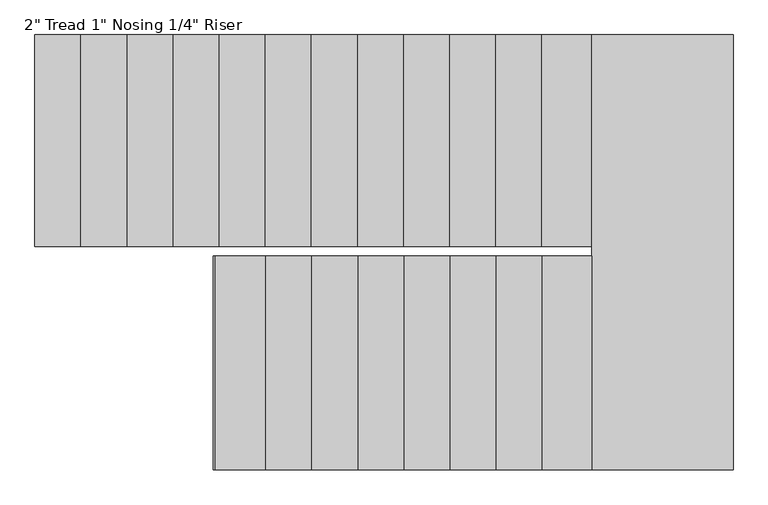
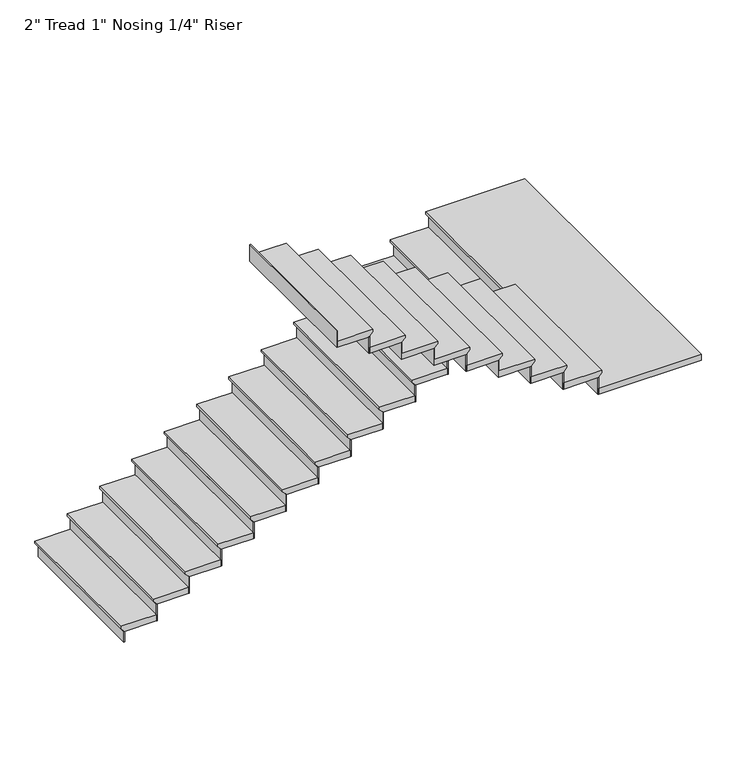
"""IFC4 building model written with IfcOpenShell, lengths in millimetres: stair flight geometry."""

from ifc_helpers import new_model, si_unit, origin, place, context, project, spatial, faceted_brep, source, transform, mapped, element, save


def stair_flight_0bd31da3(model_context):
    return source(origin(), model_context, "Body", "Brep", [
        faceted_brep([(1811.8890963, 296.3962251, 15359.4954545), (1811.8890963, 296.3962251, 15378.5454545), (1811.8890963, 1464.7962251, 15378.5454545), (1811.8890963, 1464.7962251, 15359.4954545), (1837.2890963, 296.3962251, 15334.0954545), (1837.2890963, 1464.7962251, 15334.0954545), (2091.2890963, 296.3962251, 15378.5454545), (2091.2890963, 1464.7962251, 15378.5454545), (1837.2890963, 1464.7962251, 15327.7454545), (2091.2890963, 1464.7962251, 15327.7454545), (2091.2890963, 296.3962251, 15327.7454545), (1837.2890963, 296.3962251, 15327.7454545)], [[[0, 1, 2, 3]], [[4, 0, 3, 5]], [[2, 1, 6, 7]], [[8, 9, 10, 11]], [[2, 7, 9, 8, 5, 3]], [[8, 11, 4, 5]], [[6, 1, 0, 4, 11, 10]], [[7, 6, 10, 9]]]),
        faceted_brep([(1837.2890963, 296.3962251, 15327.7454545), (1837.2890963, 296.3962251, 15240.0), (1843.6390963, 296.3962251, 15240.0), (1843.6390963, 296.3962251, 15327.7454545), (1837.2890963, 1464.7962251, 15327.7454545), (1843.6390963, 1464.7962251, 15327.7454545), (1843.6390963, 1464.7962251, 15240.0), (1837.2890963, 1464.7962251, 15240.0)], [[[0, 1, 2, 3]], [[4, 5, 6, 7]], [[1, 0, 4, 7]], [[2, 1, 7, 6]], [[3, 2, 6, 5]], [[0, 3, 5, 4]]]),
        faceted_brep([(2091.2890963, 296.3962251, 15466.2909091), (2091.2890963, 296.3962251, 15327.7454545), (2097.6390963, 296.3962251, 15327.7454545), (2097.6390963, 296.3962251, 15466.2909091), (2091.2890963, 1464.7962251, 15466.2909091), (2097.6390963, 1464.7962251, 15466.2909091), (2097.6390963, 1464.7962251, 15327.7454545), (2091.2890963, 1464.7962251, 15327.7454545)], [[[0, 1, 2, 3]], [[4, 5, 6, 7]], [[1, 0, 4, 7]], [[2, 1, 7, 6]], [[3, 2, 6, 5]], [[0, 3, 5, 4]]]),
        faceted_brep([(2065.8890963, 1464.7962251, 15517.0909091), (2065.8890963, 296.3962251, 15517.0909091), (2345.2890963, 296.3962251, 15517.0909091), (2345.2890963, 1464.7962251, 15517.0909091), (2091.2890963, 1464.7962251, 15466.2909091), (2345.2890963, 1464.7962251, 15466.2909091), (2345.2890963, 296.3962251, 15466.2909091), (2091.2890963, 296.3962251, 15466.2909091), (2091.2890963, 1464.7962251, 15472.6409091), (2065.8890963, 1464.7962251, 15498.0409091), (2091.2890963, 296.3962251, 15472.6409091), (2065.8890963, 296.3962251, 15498.0409091)], [[[0, 1, 2, 3]], [[4, 5, 6, 7]], [[0, 3, 5, 4, 8, 9]], [[4, 7, 10, 8]], [[2, 1, 11, 10, 7, 6]], [[3, 2, 6, 5]], [[11, 1, 0, 9]], [[10, 11, 9, 8]]]),
        faceted_brep([(2345.2890963, 296.3962251, 15604.8363636), (2345.2890963, 296.3962251, 15466.2909091), (2351.6390963, 296.3962251, 15466.2909091), (2351.6390963, 296.3962251, 15604.8363636), (2345.2890963, 1464.7962251, 15604.8363636), (2351.6390963, 1464.7962251, 15604.8363636), (2351.6390963, 1464.7962251, 15466.2909091), (2345.2890963, 1464.7962251, 15466.2909091)], [[[0, 1, 2, 3]], [[4, 5, 6, 7]], [[1, 0, 4, 7]], [[2, 1, 7, 6]], [[3, 2, 6, 5]], [[0, 3, 5, 4]]]),
        faceted_brep([(2319.8890963, 1464.7962251, 15655.6363636), (2319.8890963, 296.3962251, 15655.6363636), (2599.2890963, 296.3962251, 15655.6363636), (2599.2890963, 1464.7962251, 15655.6363636), (2345.2890963, 1464.7962251, 15604.8363636), (2599.2890963, 1464.7962251, 15604.8363636), (2599.2890963, 296.3962251, 15604.8363636), (2345.2890963, 296.3962251, 15604.8363636), (2345.2890963, 1464.7962251, 15611.1863636), (2319.8890963, 1464.7962251, 15636.5863636), (2345.2890963, 296.3962251, 15611.1863636), (2319.8890963, 296.3962251, 15636.5863636)], [[[0, 1, 2, 3]], [[4, 5, 6, 7]], [[0, 3, 5, 4, 8, 9]], [[4, 7, 10, 8]], [[2, 1, 11, 10, 7, 6]], [[3, 2, 6, 5]], [[11, 1, 0, 9]], [[10, 11, 9, 8]]]),
        faceted_brep([(2599.2890963, 296.3962251, 15743.3818182), (2599.2890963, 296.3962251, 15604.8363636), (2605.6390963, 296.3962251, 15604.8363636), (2605.6390963, 296.3962251, 15743.3818182), (2599.2890963, 1464.7962251, 15743.3818182), (2605.6390963, 1464.7962251, 15743.3818182), (2605.6390963, 1464.7962251, 15604.8363636), (2599.2890963, 1464.7962251, 15604.8363636)], [[[0, 1, 2, 3]], [[4, 5, 6, 7]], [[1, 0, 4, 7]], [[2, 1, 7, 6]], [[3, 2, 6, 5]], [[0, 3, 5, 4]]]),
        faceted_brep([(2573.8890963, 1464.7962251, 15794.1818182), (2573.8890963, 296.3962251, 15794.1818182), (2853.2890963, 296.3962251, 15794.1818182), (2853.2890963, 1464.7962251, 15794.1818182), (2599.2890963, 1464.7962251, 15743.3818182), (2853.2890963, 1464.7962251, 15743.3818182), (2853.2890963, 296.3962251, 15743.3818182), (2599.2890963, 296.3962251, 15743.3818182), (2599.2890963, 1464.7962251, 15749.7318182), (2573.8890963, 1464.7962251, 15775.1318182), (2599.2890963, 296.3962251, 15749.7318182), (2573.8890963, 296.3962251, 15775.1318182)], [[[0, 1, 2, 3]], [[4, 5, 6, 7]], [[0, 3, 5, 4, 8, 9]], [[4, 7, 10, 8]], [[2, 1, 11, 10, 7, 6]], [[3, 2, 6, 5]], [[11, 1, 0, 9]], [[10, 11, 9, 8]]]),
        faceted_brep([(2853.2890963, 296.3962251, 15881.9272727), (2853.2890963, 296.3962251, 15743.3818182), (2859.6390963, 296.3962251, 15743.3818182), (2859.6390963, 296.3962251, 15881.9272727), (2853.2890963, 1464.7962251, 15881.9272727), (2859.6390963, 1464.7962251, 15881.9272727), (2859.6390963, 1464.7962251, 15743.3818182), (2853.2890963, 1464.7962251, 15743.3818182)], [[[0, 1, 2, 3]], [[4, 5, 6, 7]], [[1, 0, 4, 7]], [[2, 1, 7, 6]], [[3, 2, 6, 5]], [[0, 3, 5, 4]]]),
        faceted_brep([(2827.8890963, 1464.7962251, 15932.7272727), (2827.8890963, 296.3962251, 15932.7272727), (3107.2890963, 296.3962251, 15932.7272727), (3107.2890963, 1464.7962251, 15932.7272727), (2853.2890963, 1464.7962251, 15881.9272727), (3107.2890963, 1464.7962251, 15881.9272727), (3107.2890963, 296.3962251, 15881.9272727), (2853.2890963, 296.3962251, 15881.9272727), (2853.2890963, 1464.7962251, 15888.2772727), (2827.8890963, 1464.7962251, 15913.6772727), (2853.2890963, 296.3962251, 15888.2772727), (2827.8890963, 296.3962251, 15913.6772727)], [[[0, 1, 2, 3]], [[4, 5, 6, 7]], [[0, 3, 5, 4, 8, 9]], [[4, 7, 10, 8]], [[2, 1, 11, 10, 7, 6]], [[3, 2, 6, 5]], [[11, 1, 0, 9]], [[10, 11, 9, 8]]]),
        faceted_brep([(3107.2890963, 296.3962251, 16020.4727273), (3107.2890963, 296.3962251, 15881.9272727), (3113.6390963, 296.3962251, 15881.9272727), (3113.6390963, 296.3962251, 16020.4727273), (3107.2890963, 1464.7962251, 16020.4727273), (3113.6390963, 1464.7962251, 16020.4727273), (3113.6390963, 1464.7962251, 15881.9272727), (3107.2890963, 1464.7962251, 15881.9272727)], [[[0, 1, 2, 3]], [[4, 5, 6, 7]], [[1, 0, 4, 7]], [[2, 1, 7, 6]], [[3, 2, 6, 5]], [[0, 3, 5, 4]]]),
        faceted_brep([(3081.8890963, 1464.7962251, 16071.2727273), (3081.8890963, 296.3962251, 16071.2727273), (3361.2890963, 296.3962251, 16071.2727273), (3361.2890963, 1464.7962251, 16071.2727273), (3107.2890963, 1464.7962251, 16020.4727273), (3361.2890963, 1464.7962251, 16020.4727273), (3361.2890963, 296.3962251, 16020.4727273), (3107.2890963, 296.3962251, 16020.4727273), (3107.2890963, 1464.7962251, 16026.8227273), (3081.8890963, 1464.7962251, 16052.2227273), (3107.2890963, 296.3962251, 16026.8227273), (3081.8890963, 296.3962251, 16052.2227273)], [[[0, 1, 2, 3]], [[4, 5, 6, 7]], [[0, 3, 5, 4, 8, 9]], [[4, 7, 10, 8]], [[2, 1, 11, 10, 7, 6]], [[3, 2, 6, 5]], [[11, 1, 0, 9]], [[10, 11, 9, 8]]]),
        faceted_brep([(3361.2890963, 296.3962251, 16159.0181818), (3361.2890963, 296.3962251, 16020.4727273), (3367.6390963, 296.3962251, 16020.4727273), (3367.6390963, 296.3962251, 16159.0181818), (3361.2890963, 1464.7962251, 16159.0181818), (3367.6390963, 1464.7962251, 16159.0181818), (3367.6390963, 1464.7962251, 16020.4727273), (3361.2890963, 1464.7962251, 16020.4727273)], [[[0, 1, 2, 3]], [[4, 5, 6, 7]], [[1, 0, 4, 7]], [[2, 1, 7, 6]], [[3, 2, 6, 5]], [[0, 3, 5, 4]]]),
        faceted_brep([(3335.8890963, 1464.7962251, 16209.8181818), (3335.8890963, 296.3962251, 16209.8181818), (3615.2890963, 296.3962251, 16209.8181818), (3615.2890963, 1464.7962251, 16209.8181818), (3361.2890963, 1464.7962251, 16159.0181818), (3615.2890963, 1464.7962251, 16159.0181818), (3615.2890963, 296.3962251, 16159.0181818), (3361.2890963, 296.3962251, 16159.0181818), (3361.2890963, 1464.7962251, 16165.3681818), (3335.8890963, 1464.7962251, 16190.7681818), (3361.2890963, 296.3962251, 16165.3681818), (3335.8890963, 296.3962251, 16190.7681818)], [[[0, 1, 2, 3]], [[4, 5, 6, 7]], [[0, 3, 5, 4, 8, 9]], [[4, 7, 10, 8]], [[2, 1, 11, 10, 7, 6]], [[3, 2, 6, 5]], [[11, 1, 0, 9]], [[10, 11, 9, 8]]]),
        faceted_brep([(3615.2890963, 296.3962251, 16297.5636364), (3615.2890963, 296.3962251, 16159.0181818), (3621.6390963, 296.3962251, 16159.0181818), (3621.6390963, 296.3962251, 16297.5636364), (3615.2890963, 1464.7962251, 16297.5636364), (3621.6390963, 1464.7962251, 16297.5636364), (3621.6390963, 1464.7962251, 16159.0181818), (3615.2890963, 1464.7962251, 16159.0181818)], [[[0, 1, 2, 3]], [[4, 5, 6, 7]], [[1, 0, 4, 7]], [[2, 1, 7, 6]], [[3, 2, 6, 5]], [[0, 3, 5, 4]]]),
        faceted_brep([(3589.8890963, 1464.7962251, 16348.3636364), (3589.8890963, 296.3962251, 16348.3636364), (3869.2890963, 296.3962251, 16348.3636364), (3869.2890963, 1464.7962251, 16348.3636364), (3615.2890963, 1464.7962251, 16297.5636364), (3869.2890963, 1464.7962251, 16297.5636364), (3869.2890963, 296.3962251, 16297.5636364), (3615.2890963, 296.3962251, 16297.5636364), (3615.2890963, 1464.7962251, 16303.9136364), (3589.8890963, 1464.7962251, 16329.3136364), (3615.2890963, 296.3962251, 16303.9136364), (3589.8890963, 296.3962251, 16329.3136364)], [[[0, 1, 2, 3]], [[4, 5, 6, 7]], [[0, 3, 5, 4, 8, 9]], [[4, 7, 10, 8]], [[2, 1, 11, 10, 7, 6]], [[3, 2, 6, 5]], [[11, 1, 0, 9]], [[10, 11, 9, 8]]]),
        faceted_brep([(3869.2890963, 296.3962251, 16436.1090909), (3869.2890963, 296.3962251, 16297.5636364), (3875.6390963, 296.3962251, 16297.5636364), (3875.6390963, 296.3962251, 16436.1090909), (3869.2890963, 1464.7962251, 16436.1090909), (3875.6390963, 1464.7962251, 16436.1090909), (3875.6390963, 1464.7962251, 16297.5636364), (3869.2890963, 1464.7962251, 16297.5636364)], [[[0, 1, 2, 3]], [[4, 5, 6, 7]], [[1, 0, 4, 7]], [[2, 1, 7, 6]], [[3, 2, 6, 5]], [[0, 3, 5, 4]]]),
        faceted_brep([(3843.8890963, 1464.7962251, 16486.9090909), (3843.8890963, 296.3962251, 16486.9090909), (4123.2890963, 296.3962251, 16486.9090909), (4123.2890963, 1464.7962251, 16486.9090909), (3869.2890963, 1464.7962251, 16436.1090909), (4123.2890963, 1464.7962251, 16436.1090909), (4123.2890963, 296.3962251, 16436.1090909), (3869.2890963, 296.3962251, 16436.1090909), (3869.2890963, 1464.7962251, 16442.4590909), (3843.8890963, 1464.7962251, 16467.8590909), (3869.2890963, 296.3962251, 16442.4590909), (3843.8890963, 296.3962251, 16467.8590909)], [[[0, 1, 2, 3]], [[4, 5, 6, 7]], [[0, 3, 5, 4, 8, 9]], [[4, 7, 10, 8]], [[2, 1, 11, 10, 7, 6]], [[3, 2, 6, 5]], [[11, 1, 0, 9]], [[10, 11, 9, 8]]]),
        faceted_brep([(4123.2890963, 296.3962251, 16574.6545455), (4123.2890963, 296.3962251, 16436.1090909), (4129.6390963, 296.3962251, 16436.1090909), (4129.6390963, 296.3962251, 16574.6545455), (4123.2890963, 1464.7962251, 16574.6545455), (4129.6390963, 1464.7962251, 16574.6545455), (4129.6390963, 1464.7962251, 16436.1090909), (4123.2890963, 1464.7962251, 16436.1090909)], [[[0, 1, 2, 3]], [[4, 5, 6, 7]], [[1, 0, 4, 7]], [[2, 1, 7, 6]], [[3, 2, 6, 5]], [[0, 3, 5, 4]]]),
        faceted_brep([(4097.8890963, 1464.7962251, 16625.4545455), (4097.8890963, 296.3962251, 16625.4545455), (4377.2890963, 296.3962251, 16625.4545455), (4377.2890963, 1464.7962251, 16625.4545455), (4123.2890963, 1464.7962251, 16574.6545455), (4377.2890963, 1464.7962251, 16574.6545455), (4377.2890963, 296.3962251, 16574.6545455), (4123.2890963, 296.3962251, 16574.6545455), (4123.2890963, 1464.7962251, 16581.0045455), (4097.8890963, 1464.7962251, 16606.4045455), (4123.2890963, 296.3962251, 16581.0045455), (4097.8890963, 296.3962251, 16606.4045455)], [[[0, 1, 2, 3]], [[4, 5, 6, 7]], [[0, 3, 5, 4, 8, 9]], [[4, 7, 10, 8]], [[2, 1, 11, 10, 7, 6]], [[3, 2, 6, 5]], [[11, 1, 0, 9]], [[10, 11, 9, 8]]]),
        faceted_brep([(4377.2890963, 296.3962251, 16713.2), (4377.2890963, 296.3962251, 16574.6545455), (4383.6390963, 296.3962251, 16574.6545455), (4383.6390963, 296.3962251, 16713.2), (4377.2890963, 1464.7962251, 16713.2), (4383.6390963, 1464.7962251, 16713.2), (4383.6390963, 1464.7962251, 16574.6545455), (4377.2890963, 1464.7962251, 16574.6545455)], [[[0, 1, 2, 3]], [[4, 5, 6, 7]], [[1, 0, 4, 7]], [[2, 1, 7, 6]], [[3, 2, 6, 5]], [[0, 3, 5, 4]]]),
        faceted_brep([(4351.8890963, 1464.7962251, 16764.0), (4351.8890963, 296.3962251, 16764.0), (4631.2890963, 296.3962251, 16764.0), (4631.2890963, 1464.7962251, 16764.0), (4377.2890963, 1464.7962251, 16713.2), (4631.2890963, 1464.7962251, 16713.2), (4631.2890963, 296.3962251, 16713.2), (4377.2890963, 296.3962251, 16713.2), (4377.2890963, 1464.7962251, 16719.55), (4351.8890963, 1464.7962251, 16744.95), (4377.2890963, 296.3962251, 16719.55), (4351.8890963, 296.3962251, 16744.95)], [[[0, 1, 2, 3]], [[4, 5, 6, 7]], [[0, 3, 5, 4, 8, 9]], [[4, 7, 10, 8]], [[2, 1, 11, 10, 7, 6]], [[3, 2, 6, 5]], [[11, 1, 0, 9]], [[10, 11, 9, 8]]]),
        faceted_brep([(4631.2890963, 296.3962251, 16851.7454545), (4631.2890963, 296.3962251, 16713.2), (4637.6390963, 296.3962251, 16713.2), (4637.6390963, 296.3962251, 16851.7454545), (4631.2890963, 1464.7962251, 16851.7454545), (4637.6390963, 1464.7962251, 16851.7454545), (4637.6390963, 1464.7962251, 16713.2), (4631.2890963, 1464.7962251, 16713.2)], [[[0, 1, 2, 3]], [[4, 5, 6, 7]], [[1, 0, 4, 7]], [[2, 1, 7, 6]], [[3, 2, 6, 5]], [[0, 3, 5, 4]]]),
        faceted_brep([(4605.8890963, 1464.7962251, 16902.5454545), (4605.8890963, 296.3962251, 16902.5454545), (4906.4326586, 296.3962251, 16902.5454545), (4906.4326586, 1464.7962251, 16902.5454545), (4631.2890963, 1464.7962251, 16851.7454545), (4906.4326586, 1464.7962251, 16851.7454545), (4906.4326586, 296.3962251, 16851.7454545), (4631.2890963, 296.3962251, 16851.7454545), (4631.2890963, 1464.7962251, 16858.0954545), (4605.8890963, 1464.7962251, 16883.4954545), (4631.2890963, 296.3962251, 16858.0954545), (4605.8890963, 296.3962251, 16883.4954545)], [[[0, 1, 2, 3]], [[4, 5, 6, 7]], [[0, 3, 5, 4, 8, 9]], [[4, 7, 10, 8]], [[2, 1, 11, 10, 7, 6]], [[3, 2, 6, 5]], [[11, 1, 0, 9]], [[10, 11, 9, 8]]]),
        faceted_brep([(4906.4326586, 296.3962251, 16990.2909091), (4906.4326586, 296.3962251, 16851.7454545), (4912.7826586, 296.3962251, 16851.7454545), (4912.7826586, 296.3962251, 16990.2909091), (4906.4326586, 1464.7962251, 16990.2909091), (4912.7826586, 1464.7962251, 16990.2909091), (4912.7826586, 1464.7962251, 16851.7454545), (4906.4326586, 1464.7962251, 16851.7454545)], [[[0, 1, 2, 3]], [[4, 5, 6, 7]], [[1, 0, 4, 7]], [[2, 1, 7, 6]], [[3, 2, 6, 5]], [[0, 3, 5, 4]]]),
        faceted_brep([(4855.6326586, -935.5037749, 17041.0909091), (5659.9890963, -935.5037749, 17041.0909091), (5659.9890963, 1464.7962251, 17041.0909091), (4881.0326586, 1464.7962251, 17041.0909091), (4881.0326586, 245.5962251, 17041.0909091), (4855.6326586, 245.5962251, 17041.0909091), (5659.9890963, -935.5037749, 16990.2909091), (4855.6326586, -935.5037749, 16990.2909091), (4855.6326586, 245.5962251, 16990.2909091), (4881.0326586, 245.5962251, 16990.2909091), (4881.0326586, 296.3962251, 16990.2909091), (4906.4326586, 296.3962251, 16990.2909091), (4906.4326586, 1464.7962251, 16990.2909091), (5659.9890963, 1464.7962251, 16990.2909091), (4906.4326586, 1464.7962251, 16996.6409091), (4881.0326586, 1464.7962251, 17022.0409091), (4906.4326586, 296.3962251, 16996.6409091), (4881.0326586, 296.3962251, 17022.0409091)], [[[0, 1, 2, 3, 4, 5]], [[6, 7, 8, 9, 10, 11, 12, 13]], [[1, 0, 7, 6]], [[2, 1, 6, 13]], [[3, 2, 13, 12, 14, 15]], [[12, 11, 16, 14]], [[11, 10, 17, 16]], [[4, 3, 15, 17, 10, 9]], [[5, 4, 9, 8]], [[0, 5, 8, 7]], [[15, 14, 16, 17]]]),
        faceted_brep([(4855.6326586, 245.5962251, 17128.8363636), (4855.6326586, 245.5962251, 16990.2909091), (4849.2826586, 245.5962251, 16990.2909091), (4849.2826586, 245.5962251, 17128.8363636), (4855.6326586, -935.5037749, 17128.8363636), (4849.2826586, -935.5037749, 17128.8363636), (4849.2826586, -935.5037749, 16990.2909091), (4855.6326586, -935.5037749, 16990.2909091)], [[[0, 1, 2, 3]], [[4, 5, 6, 7]], [[1, 0, 4, 7]], [[2, 1, 7, 6]], [[3, 2, 6, 5]], [[0, 3, 5, 4]]]),
        faceted_brep([(4881.0326586, -935.5037749, 17179.6363636), (4881.0326586, 245.5962251, 17179.6363636), (4580.4890963, 245.5962251, 17179.6363636), (4580.4890963, -935.5037749, 17179.6363636), (4855.6326586, -935.5037749, 17128.8363636), (4580.4890963, -935.5037749, 17128.8363636), (4580.4890963, 245.5962251, 17128.8363636), (4855.6326586, 245.5962251, 17128.8363636), (4855.6326586, -935.5037749, 17135.1863636), (4881.0326586, -935.5037749, 17160.5863636), (4855.6326586, 245.5962251, 17135.1863636), (4881.0326586, 245.5962251, 17160.5863636)], [[[0, 1, 2, 3]], [[4, 5, 6, 7]], [[0, 3, 5, 4, 8, 9]], [[4, 7, 10, 8]], [[2, 1, 11, 10, 7, 6]], [[3, 2, 6, 5]], [[11, 1, 0, 9]], [[10, 11, 9, 8]]]),
        faceted_brep([(4580.4890963, 245.5962251, 17267.3818182), (4580.4890963, 245.5962251, 17128.8363636), (4574.1390963, 245.5962251, 17128.8363636), (4574.1390963, 245.5962251, 17267.3818182), (4580.4890963, -935.5037749, 17267.3818182), (4574.1390963, -935.5037749, 17267.3818182), (4574.1390963, -935.5037749, 17128.8363636), (4580.4890963, -935.5037749, 17128.8363636)], [[[0, 1, 2, 3]], [[4, 5, 6, 7]], [[1, 0, 4, 7]], [[2, 1, 7, 6]], [[3, 2, 6, 5]], [[0, 3, 5, 4]]]),
        faceted_brep([(4605.8890963, -935.5037749, 17318.1818182), (4605.8890963, 245.5962251, 17318.1818182), (4326.4890963, 245.5962251, 17318.1818182), (4326.4890963, -935.5037749, 17318.1818182), (4580.4890963, -935.5037749, 17267.3818182), (4326.4890963, -935.5037749, 17267.3818182), (4326.4890963, 245.5962251, 17267.3818182), (4580.4890963, 245.5962251, 17267.3818182), (4580.4890963, -935.5037749, 17273.7318182), (4605.8890963, -935.5037749, 17299.1318182), (4580.4890963, 245.5962251, 17273.7318182), (4605.8890963, 245.5962251, 17299.1318182)], [[[0, 1, 2, 3]], [[4, 5, 6, 7]], [[0, 3, 5, 4, 8, 9]], [[4, 7, 10, 8]], [[2, 1, 11, 10, 7, 6]], [[3, 2, 6, 5]], [[11, 1, 0, 9]], [[10, 11, 9, 8]]]),
        faceted_brep([(4326.4890963, 245.5962251, 17405.9272727), (4326.4890963, 245.5962251, 17267.3818182), (4320.1390963, 245.5962251, 17267.3818182), (4320.1390963, 245.5962251, 17405.9272727), (4326.4890963, -935.5037749, 17405.9272727), (4320.1390963, -935.5037749, 17405.9272727), (4320.1390963, -935.5037749, 17267.3818182), (4326.4890963, -935.5037749, 17267.3818182)], [[[0, 1, 2, 3]], [[4, 5, 6, 7]], [[1, 0, 4, 7]], [[2, 1, 7, 6]], [[3, 2, 6, 5]], [[0, 3, 5, 4]]]),
        faceted_brep([(4351.8890963, -935.5037749, 17456.7272727), (4351.8890963, 245.5962251, 17456.7272727), (4072.4890963, 245.5962251, 17456.7272727), (4072.4890963, -935.5037749, 17456.7272727), (4326.4890963, -935.5037749, 17405.9272727), (4072.4890963, -935.5037749, 17405.9272727), (4072.4890963, 245.5962251, 17405.9272727), (4326.4890963, 245.5962251, 17405.9272727), (4326.4890963, -935.5037749, 17412.2772727), (4351.8890963, -935.5037749, 17437.6772727), (4326.4890963, 245.5962251, 17412.2772727), (4351.8890963, 245.5962251, 17437.6772727)], [[[0, 1, 2, 3]], [[4, 5, 6, 7]], [[0, 3, 5, 4, 8, 9]], [[4, 7, 10, 8]], [[2, 1, 11, 10, 7, 6]], [[3, 2, 6, 5]], [[11, 1, 0, 9]], [[10, 11, 9, 8]]]),
        faceted_brep([(4072.4890963, 245.5962251, 17544.4727273), (4072.4890963, 245.5962251, 17405.9272727), (4066.1390963, 245.5962251, 17405.9272727), (4066.1390963, 245.5962251, 17544.4727273), (4072.4890963, -935.5037749, 17544.4727273), (4066.1390963, -935.5037749, 17544.4727273), (4066.1390963, -935.5037749, 17405.9272727), (4072.4890963, -935.5037749, 17405.9272727)], [[[0, 1, 2, 3]], [[4, 5, 6, 7]], [[1, 0, 4, 7]], [[2, 1, 7, 6]], [[3, 2, 6, 5]], [[0, 3, 5, 4]]]),
        faceted_brep([(4097.8890963, -935.5037749, 17595.2727273), (4097.8890963, 245.5962251, 17595.2727273), (3818.4890963, 245.5962251, 17595.2727273), (3818.4890963, -935.5037749, 17595.2727273), (4072.4890963, -935.5037749, 17544.4727273), (3818.4890963, -935.5037749, 17544.4727273), (3818.4890963, 245.5962251, 17544.4727273), (4072.4890963, 245.5962251, 17544.4727273), (4072.4890963, -935.5037749, 17550.8227273), (4097.8890963, -935.5037749, 17576.2227273), (4072.4890963, 245.5962251, 17550.8227273), (4097.8890963, 245.5962251, 17576.2227273)], [[[0, 1, 2, 3]], [[4, 5, 6, 7]], [[0, 3, 5, 4, 8, 9]], [[4, 7, 10, 8]], [[2, 1, 11, 10, 7, 6]], [[3, 2, 6, 5]], [[11, 1, 0, 9]], [[10, 11, 9, 8]]]),
        faceted_brep([(3818.4890963, 245.5962251, 17683.0181818), (3818.4890963, 245.5962251, 17544.4727273), (3812.1390963, 245.5962251, 17544.4727273), (3812.1390963, 245.5962251, 17683.0181818), (3818.4890963, -935.5037749, 17683.0181818), (3812.1390963, -935.5037749, 17683.0181818), (3812.1390963, -935.5037749, 17544.4727273), (3818.4890963, -935.5037749, 17544.4727273)], [[[0, 1, 2, 3]], [[4, 5, 6, 7]], [[1, 0, 4, 7]], [[2, 1, 7, 6]], [[3, 2, 6, 5]], [[0, 3, 5, 4]]]),
        faceted_brep([(3843.8890963, -935.5037749, 17733.8181818), (3843.8890963, 245.5962251, 17733.8181818), (3564.4890963, 245.5962251, 17733.8181818), (3564.4890963, -935.5037749, 17733.8181818), (3818.4890963, -935.5037749, 17683.0181818), (3564.4890963, -935.5037749, 17683.0181818), (3564.4890963, 245.5962251, 17683.0181818), (3818.4890963, 245.5962251, 17683.0181818), (3818.4890963, -935.5037749, 17689.3681818), (3843.8890963, -935.5037749, 17714.7681818), (3818.4890963, 245.5962251, 17689.3681818), (3843.8890963, 245.5962251, 17714.7681818)], [[[0, 1, 2, 3]], [[4, 5, 6, 7]], [[0, 3, 5, 4, 8, 9]], [[4, 7, 10, 8]], [[2, 1, 11, 10, 7, 6]], [[3, 2, 6, 5]], [[11, 1, 0, 9]], [[10, 11, 9, 8]]]),
        faceted_brep([(3564.4890963, 245.5962251, 17821.5636364), (3564.4890963, 245.5962251, 17683.0181818), (3558.1390963, 245.5962251, 17683.0181818), (3558.1390963, 245.5962251, 17821.5636364), (3564.4890963, -935.5037749, 17821.5636364), (3558.1390963, -935.5037749, 17821.5636364), (3558.1390963, -935.5037749, 17683.0181818), (3564.4890963, -935.5037749, 17683.0181818)], [[[0, 1, 2, 3]], [[4, 5, 6, 7]], [[1, 0, 4, 7]], [[2, 1, 7, 6]], [[3, 2, 6, 5]], [[0, 3, 5, 4]]]),
        faceted_brep([(3589.8890963, -935.5037749, 17872.3636364), (3589.8890963, 245.5962251, 17872.3636364), (3310.4890963, 245.5962251, 17872.3636364), (3310.4890963, -935.5037749, 17872.3636364), (3564.4890963, -935.5037749, 17821.5636364), (3310.4890963, -935.5037749, 17821.5636364), (3310.4890963, 245.5962251, 17821.5636364), (3564.4890963, 245.5962251, 17821.5636364), (3564.4890963, -935.5037749, 17827.9136364), (3589.8890963, -935.5037749, 17853.3136364), (3564.4890963, 245.5962251, 17827.9136364), (3589.8890963, 245.5962251, 17853.3136364)], [[[0, 1, 2, 3]], [[4, 5, 6, 7]], [[0, 3, 5, 4, 8, 9]], [[4, 7, 10, 8]], [[2, 1, 11, 10, 7, 6]], [[3, 2, 6, 5]], [[11, 1, 0, 9]], [[10, 11, 9, 8]]]),
        faceted_brep([(3310.4890963, 245.5962251, 17960.1090909), (3310.4890963, 245.5962251, 17821.5636364), (3304.1390963, 245.5962251, 17821.5636364), (3304.1390963, 245.5962251, 17960.1090909), (3310.4890963, -935.5037749, 17960.1090909), (3304.1390963, -935.5037749, 17960.1090909), (3304.1390963, -935.5037749, 17821.5636364), (3310.4890963, -935.5037749, 17821.5636364)], [[[0, 1, 2, 3]], [[4, 5, 6, 7]], [[1, 0, 4, 7]], [[2, 1, 7, 6]], [[3, 2, 6, 5]], [[0, 3, 5, 4]]]),
        faceted_brep([(3335.8890963, -935.5037749, 18010.9090909), (3335.8890963, 245.5962251, 18010.9090909), (3056.4890963, 245.5962251, 18010.9090909), (3056.4890963, -935.5037749, 18010.9090909), (3310.4890963, -935.5037749, 17960.1090909), (3056.4890963, -935.5037749, 17960.1090909), (3056.4890963, 245.5962251, 17960.1090909), (3310.4890963, 245.5962251, 17960.1090909), (3310.4890963, -935.5037749, 17966.4590909), (3335.8890963, -935.5037749, 17991.8590909), (3310.4890963, 245.5962251, 17966.4590909), (3335.8890963, 245.5962251, 17991.8590909)], [[[0, 1, 2, 3]], [[4, 5, 6, 7]], [[0, 3, 5, 4, 8, 9]], [[4, 7, 10, 8]], [[2, 1, 11, 10, 7, 6]], [[3, 2, 6, 5]], [[11, 1, 0, 9]], [[10, 11, 9, 8]]]),
        faceted_brep([(3056.4890963, 245.5962251, 18098.6545455), (3056.4890963, 245.5962251, 17960.1090909), (3050.1390963, 245.5962251, 17960.1090909), (3050.1390963, 245.5962251, 18098.6545455), (3056.4890963, -935.5037749, 18098.6545455), (3050.1390963, -935.5037749, 18098.6545455), (3050.1390963, -935.5037749, 17960.1090909), (3056.4890963, -935.5037749, 17960.1090909)], [[[0, 1, 2, 3]], [[4, 5, 6, 7]], [[1, 0, 4, 7]], [[2, 1, 7, 6]], [[3, 2, 6, 5]], [[0, 3, 5, 4]]]),
        faceted_brep([(2802.4890963, 245.5962251, 18237.2), (2802.4890963, 245.5962251, 18098.6545455), (2796.1390963, 245.5962251, 18098.6545455), (2796.1390963, 245.5962251, 18237.2), (2802.4890963, -935.5037749, 18237.2), (2796.1390963, -935.5037749, 18237.2), (2796.1390963, -935.5037749, 18098.6545455), (2802.4890963, -935.5037749, 18098.6545455)], [[[0, 1, 2, 3]], [[4, 5, 6, 7]], [[1, 0, 4, 7]], [[2, 1, 7, 6]], [[3, 2, 6, 5]], [[0, 3, 5, 4]]]),
        faceted_brep([(3081.8890963, -935.5037749, 18149.4545455), (3081.8890963, 245.5962251, 18149.4545455), (2802.4890963, 245.5962251, 18149.4545455), (2802.4890963, -935.5037749, 18149.4545455), (3056.4890963, -935.5037749, 18098.6545455), (2802.4890963, -935.5037749, 18098.6545455), (2802.4890963, 245.5962251, 18098.6545455), (3056.4890963, 245.5962251, 18098.6545455), (3056.4890963, -935.5037749, 18105.0045455), (3081.8890963, -935.5037749, 18130.4045455), (3056.4890963, 245.5962251, 18105.0045455), (3081.8890963, 245.5962251, 18130.4045455)], [[[0, 1, 2, 3]], [[4, 5, 6, 7]], [[0, 3, 5, 4, 8, 9]], [[4, 7, 10, 8]], [[2, 1, 11, 10, 7, 6]], [[3, 2, 6, 5]], [[11, 1, 0, 9]], [[10, 11, 9, 8]]]),
    ])


if __name__ == "__main__":
    model = new_model("IFC4")
    model_context = context("Model", 3, world=origin())
    ifc_project = project(units=[si_unit("LENGTHUNIT", "METRE", prefix="MILLI")], contexts=[model_context])
    site = spatial("IfcSite", under=ifc_project)
    building = spatial("IfcBuilding", under=site)
    placement = place(None, origin())
    stair_flight_shape = stair_flight_0bd31da3(model_context)
    element("IfcStairFlight", 1, ObjectType="2\" Tread 1\" Nosing 1/4\" Riser", at=placement, inside=building, context=model_context, shape_type="MappedRepresentation", body=[
        mapped(stair_flight_shape, transform((0.0, 0.0, 0.0), x_axis=(1.0, 0.0, 0.0), y_axis=(0.0, 1.0, 0.0), z_axis=(0.0, 0.0, 1.0))),
    ])
    save(model, "model.ifc")
